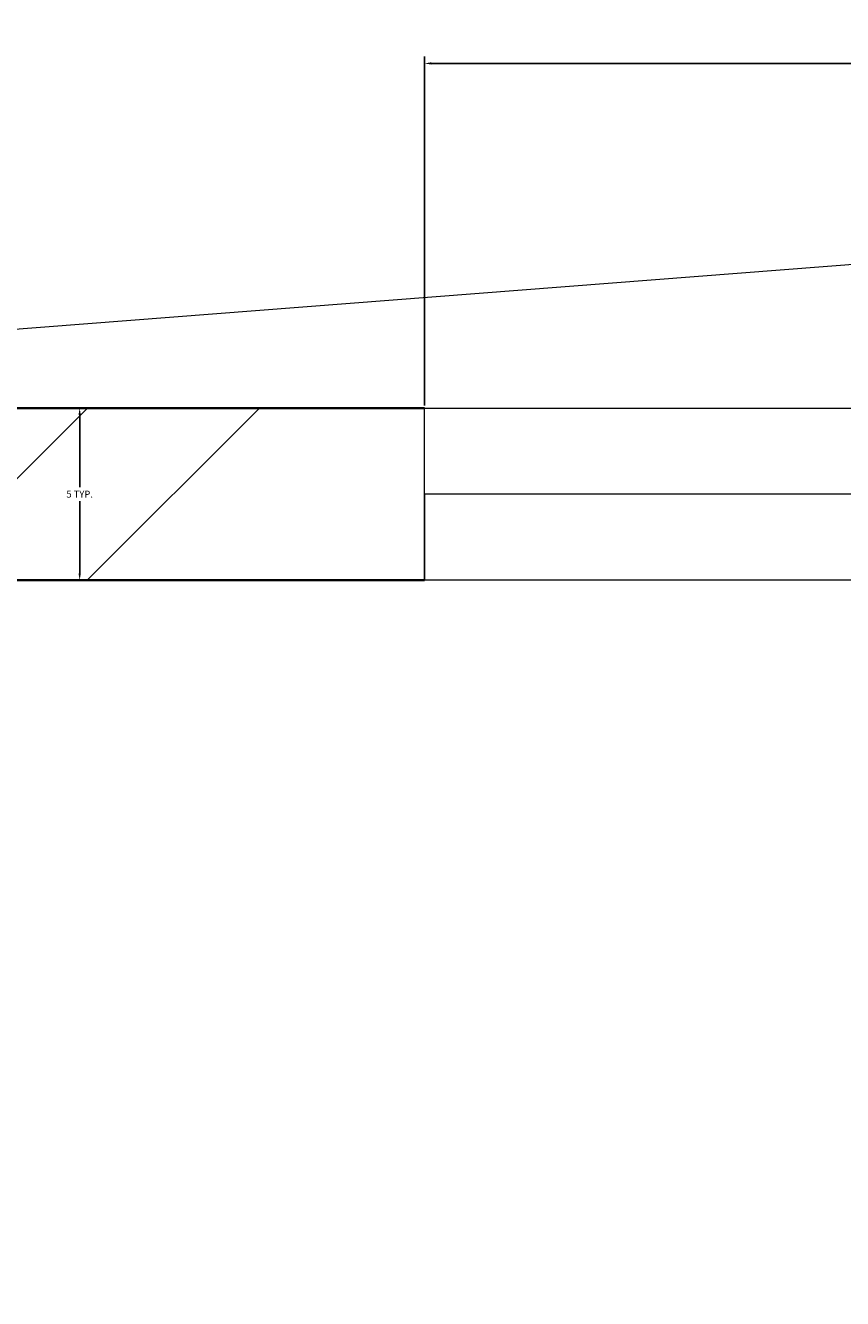
# Model space of a CAD drawing. Units: inches. Extents: x 1885 to 2748, y 783 to 2421.
# Tile 37 of 117: x 2034 to 2056, y 1501 to 1534. Entities that reach past the tile are written whole.
import ezdxf

# ---------------------------------------------------------------- set-up
doc = ezdxf.new("R2010")
doc.units = ezdxf.units.IN
for name, color, linetype, lineweight in [('A-ANNO-DIMS', 2, 'Continuous', 18), ('A-FLOR-OPEN', 8, 'Continuous', 13), ('A-GLAZ', 181, 'Continuous', 18), ('A-WALL', 7, 'Continuous', 35)]:
    doc.layers.add(name, color=color, linetype=linetype, lineweight=lineweight)
doc.layers.add('A-WALL-PATT', color=85, linetype='Continuous', lineweight=13, true_color=0x58ba48)
doc.styles.get("Standard").update_dxf_attribs({"font": 'arial.ttf'})
doc.dimstyles.get("Standard").update_dxf_attribs({"dimtxt": 0.18, "dimasz": 0.18, "dimexe": 0.18, "dimexo": 0.0625, "dimgap": 0.09, "dimtad": 0, "dimtih": 1, "dimtoh": 1, "dimdec": 4, "dimzin": 0, "dimdsep": 46, "dimtxsty": 'Standard', "dimcen": 0.09, "dimadec": 0, "dimazin": 0, "dimtfac": 1, "dimtdec": 4, "dimtofl": 0, "dimtmove": 0, "dimatfit": 3, "dimfxl": 1, "dimtolj": 1, "dimtzin": 0, "dimarcsym": 0})

# ---------------------------------------------------------------- blocks, each defined once
blk = doc.blocks.new('WIN-60')
for p, q in [((0.004, 59.998), (0.004, -0.002)), ((2.254, 59.998), (2.254, -0.002)), ((4.504, -0.002), (4.504, 59.998)), ((2.254, -0.002), (0.004, -0.002)), ((0.004, -0.002), (4.504, -0.002))]:
    blk.add_line(p, q)
blk = doc.blocks.new('*D15')
at = {"layer": 'A-ANNO-DIMS', "color": 0, "lineweight": -2, "transparency": 16777216}
for p, q in [((2044.674, 1524.068), (2044.674, 1533.186)), ((2104.674, 1524.068), (2104.674, 1533.186)), ((2044.854, 1533.006), (2073.556, 1533.006)), ((2104.494, 1533.006), (2075.793, 1533.006))]:
    blk.add_line(p, q, dxfattribs=at)
at = {"layer": 'A-ANNO-DIMS', "color": 0, "transparency": 16777216}
for points in [[(2044.854, 1533.036), (2044.854, 1532.976), (2044.674, 1533.006)], [(2104.494, 1533.036), (2104.494, 1532.976), (2104.674, 1533.006)]]:
    blk.add_solid(points, dxfattribs=at)
at = {"layer": 'Defpoints', "color": 0, "transparency": 16777216}
for p in [(2104.674, 1533.006), (2044.674, 1524.006), (2104.674, 1524.006)]:
    blk.add_point(p, dxfattribs=at)
at = {"layer": 'A-ANNO-DIMS', "color": 0, "transparency": 16777216, "insert": (2074.674, 1533.006), "char_height": 0.18, "attachment_point": 5}
blk.add_mtext('\\A1;WINDOW 60 TYP.', dxfattribs=at)
blk = doc.blocks.new('*D16')
at = {"layer": 'A-ANNO-DIMS', "color": 0, "lineweight": -2, "transparency": 16777216}
for p, q in [((2044.612, 1524.006), (2035.494, 1524.006)), ((2035.674, 1523.826), (2035.674, 1521.937)), ((2035.674, 1519.686), (2035.674, 1521.574)), ((2044.612, 1519.506), (2035.494, 1519.506))]:
    blk.add_line(p, q, dxfattribs=at)
at = {"layer": 'A-ANNO-DIMS', "color": 0, "transparency": 16777216}
for points in [[(2035.644, 1523.826), (2035.704, 1523.826), (2035.674, 1524.006)], [(2035.644, 1519.686), (2035.704, 1519.686), (2035.674, 1519.506)]]:
    blk.add_solid(points, dxfattribs=at)
at = {"layer": 'Defpoints', "color": 0, "transparency": 16777216}
for p in [(2035.674, 1524.006), (2044.674, 1524.006), (2044.674, 1519.506)]:
    blk.add_point(p, dxfattribs=at)
at = {"layer": 'A-ANNO-DIMS', "color": 0, "transparency": 16777216, "insert": (2035.674, 1521.756), "char_height": 0.18, "attachment_point": 5}
blk.add_mtext('\\A1;5 TYP.', dxfattribs=at)

msp = doc.modelspace()

# ---------------------------------------------------------------- hatches: boundary and pattern name
at = {"layer": 'A-WALL-PATT'}
h = msp.add_hatch(dxfattribs=at)
h.set_pattern_fill('ANSI32', color=256)
h.paths.add_polyline_path([(2007.772, 2318.006), (1980.774, 2318.006), (1980.774, 2281.215), (1985.274, 2281.215), (1985.274, 2313.506), (2007.772, 2313.506), (2007.772, 2315.756)])
h.paths.add_polyline_path([(2094.324, 2318.006), (2067.772, 2318.006), (2067.772, 2313.506), (2094.324, 2313.506), (2094.324, 2315.756)])
h.paths.add_polyline_path([(2131.367, 2315.756), (2131.367, 2318.006), (2131.189, 2318.006), (2112.609, 2318.006), (2112.609, 2313.506), (2117.274, 2313.506), (2117.274, 2255.201), (2121.774, 2255.201), (2121.774, 2313.506), (2131.367, 2313.506)])
h.paths.add_polyline_path([(2190.512, 2318.006), (2155.367, 2318.006), (2155.367, 2313.506), (2169.774, 2313.506), (2169.774, 2229.506), (2121.774, 2229.506), (2121.774, 2233.451), (2119.524, 2233.451), (2117.274, 2233.451), (2117.274, 2201.101), (2121.774, 2201.101), (2121.774, 2225.006), (2169.774, 2225.006), (2169.774, 2165.006), (2306.274, 2165.006), (2306.274, 2066.006), (2310.774, 2066.006), (2344.274, 2066.006), (2486.274, 2066.006), (2486.274, 1886.006), (2483.02, 1886.006), (2483.02, 1881.506), (2486.274, 1881.506), (2486.274, 1880.678), (2490.774, 1880.678), (2490.774, 2070.506), (2344.274, 2070.506), (2310.774, 2070.506), (2310.774, 2165.006), (2310.774, 2173.636), (2308.524, 2173.636), (2306.274, 2173.636), (2306.274, 2169.506), (2174.274, 2169.506), (2174.274, 2313.506), (2190.512, 2313.506), (2190.512, 2315.756)])
h.paths.add_polyline_path([(1985.274, 2221.215), (1980.774, 2221.215), (1980.774, 2165.006), (1992.774, 2165.006), (1992.774, 2141.927), (1997.274, 2141.927), (1997.274, 2165.006), (2117.274, 2165.006), (2117.274, 2163.126), (2121.774, 2163.126), (2121.774, 2172.734), (2119.524, 2172.734), (2117.274, 2172.734), (2117.274, 2169.506), (1985.274, 2169.506)])
h.paths.add_polyline_path([(1997.274, 2105.927), (1992.774, 2105.927), (1992.774, 2070.506), (2016.774, 2070.506), (2016.774, 2059.123), (2019.024, 2059.123), (2021.274, 2059.123), (2021.274, 2070.506), (2117.274, 2070.506), (2117.274, 2022.506), (2114.423, 2022.506), (2114.423, 2018.006), (2123.627, 2018.006), (2123.627, 2020.256), (2123.627, 2022.506), (2121.774, 2022.506), (2121.774, 2142.587), (2119.524, 2142.587), (2117.274, 2142.587), (2117.274, 2075.006), (1997.274, 2075.006)])
h.paths.add_polyline_path([(2092.029, 2020.256), (2092.029, 2022.506), (2021.274, 2022.506), (2021.274, 2035.123), (2016.774, 2035.123), (2016.774, 2018.006), (2016.774, 1978.784), (2021.274, 1978.784), (2021.274, 2018.006), (2092.029, 2018.006)])
h.paths.add_polyline_path([(2260.938, 2022.506), (2153.105, 2022.506), (2153.105, 2020.256), (2153.105, 2018.006), (2155.274, 2018.006), (2155.274, 1886.006), (2107.629, 1886.006), (2107.629, 1881.506), (2182.911, 1881.506), (2182.911, 1883.756), (2182.911, 1886.006), (2159.774, 1886.006), (2159.774, 2018.006), (2260.938, 2018.006), (2260.938, 2020.256)])
h.paths.add_polyline_path([(2047.629, 1883.756), (2047.629, 1886.006), (2021.274, 1886.006), (2021.274, 1918.784), (2019.024, 1918.784), (2016.774, 1918.784), (2016.774, 1881.506), (2047.629, 1881.506)])
h.paths.add_polyline_path([(2306.361, 1883.756), (2306.361, 1886.006), (2296.274, 1886.006), (2296.274, 1982.006), (2316.535, 1982.006), (2316.535, 1984.256), (2316.535, 1986.506), (2296.274, 1986.506), (2296.274, 2022.506), (2289.276, 2022.506), (2289.276, 2018.006), (2291.774, 2018.006), (2291.774, 1886.006), (2242.911, 1886.006), (2242.911, 1881.506), (2306.361, 1881.506)], flags=17)
h.paths.add_polyline_path([(1985.274, 1843.006), (2021.6, 1843.006), (2021.534, 1845.441), (2021.477, 1847.506), (1980.774, 1847.506), (1980.774, 1809.446), (1985.274, 1809.446)])
h.paths.add_polyline_path([(2131.482, 1845.256), (2131.482, 1847.506), (2081.534, 1847.506), (2081.534, 1843.006), (2117.274, 1843.006), (2117.274, 1784.147), (2119.524, 1784.147), (2121.774, 1784.147), (2121.774, 1843.006), (2131.482, 1843.006)])
h.paths.add_polyline_path([(2203.886, 1847.506), (2155.482, 1847.506), (2155.482, 1843.006), (2169.774, 1843.006), (2169.774, 1759.006), (2121.774, 1759.006), (2121.774, 1761.457), (2117.274, 1761.457), (2117.274, 1730.429), (2121.774, 1730.429), (2121.774, 1754.506), (2177.421, 1754.506), (2177.421, 1756.756), (2177.421, 1759.006), (2174.274, 1759.006), (2174.274, 1843.006), (2203.886, 1843.006)])
h.paths.add_polyline_path([(2335.554, 1845.256), (2335.554, 1847.506), (2239.886, 1847.506), (2239.886, 1843.006), (2306.274, 1843.006), (2306.274, 1759.006), (2199.486, 1759.006), (2199.486, 1754.506), (2310.774, 1754.506), (2310.774, 1843.006), (2335.554, 1843.006)])
h.paths.add_polyline_path([(2348.774, 2022.506), (2344.274, 2022.506), (2344.274, 1986.506), (2341.681, 1986.506), (2341.681, 1982.006), (2344.274, 1982.006), (2344.274, 1886.006), (2330.361, 1886.006), (2330.361, 1881.506), (2361.627, 1881.506), (2361.627, 1883.756), (2361.627, 1886.006), (2348.774, 1886.006)], flags=17)
h.paths.add_polyline_path([(2283.251, 2315.756), (2283.251, 2318.006), (2238.512, 2318.006), (2238.512, 2313.506), (2283.251, 2313.506)], flags=17)
h.paths.add_polyline_path([(2363.274, 2348.006), (2388.677, 2348.006), (2388.677, 2350.256), (2388.677, 2352.506), (2358.774, 2352.506), (2358.774, 2348.006), (2358.774, 2318.006), (2344.481, 2318.006), (2344.481, 2313.506), (2358.774, 2313.506), (2358.774, 2229.506), (2310.774, 2229.506), (2310.774, 2231.952), (2306.274, 2231.952), (2306.274, 2205.611), (2310.774, 2205.611), (2310.774, 2225.006), (2358.774, 2225.006), (2358.774, 2211.506), (2452.329, 2211.506), (2452.329, 2213.756), (2452.329, 2216.006), (2363.274, 2216.006), (2363.274, 2318.006)])
h.paths.add_polyline_path([(2310.774, 2313.506), (2320.481, 2313.506), (2320.481, 2315.756), (2320.481, 2318.006), (2302.728, 2318.006), (2302.728, 2313.506), (2306.274, 2313.506), (2306.274, 2251.076), (2310.774, 2251.076)], flags=17)
h.paths.add_polyline_path([(2490.774, 2352.506), (2486.274, 2352.506), (2448.677, 2352.506), (2448.677, 2348.006), (2486.274, 2348.006), (2486.274, 2318.006), (2486.274, 2216.006), (2481.78, 2216.006), (2481.78, 2211.506), (2486.274, 2211.506), (2486.274, 2165.006), (2493.289, 2165.006), (2493.289, 2167.256), (2493.289, 2169.506), (2490.774, 2169.506), (2490.774, 2313.506), (2494.429, 2313.506), (2494.429, 2318.006), (2490.774, 2318.006)])
h.paths.add_polyline_path([(2534.653, 2318.006), (2515.691, 2318.006), (2515.691, 2313.506), (2534.653, 2313.506), (2534.653, 2315.756)])
h.paths.add_polyline_path([(2618.274, 2318.006), (2594.653, 2318.006), (2594.653, 2313.506), (2613.774, 2313.506), (2613.774, 2281.706), (2618.274, 2281.706)])
h.paths.add_polyline_path([(2618.274, 2221.706), (2613.774, 2221.706), (2613.774, 2169.506), (2554.019, 2169.506), (2554.019, 2165.006), (2613.774, 2165.006), (2613.774, 2152.878), (2618.274, 2152.878)])
h.paths.add_polyline_path([(2618.274, 2128.878), (2616.024, 2128.878), (2613.774, 2128.878), (2613.774, 2117.006), (2529.774, 2117.006), (2529.774, 2165.006), (2532.848, 2165.006), (2532.848, 2169.506), (2522.867, 2169.506), (2522.867, 2165.006), (2525.274, 2165.006), (2525.274, 2117.006), (2525.274, 2112.506), (2525.274, 2108.576), (2529.774, 2108.576), (2529.774, 2112.506), (2613.774, 2112.506), (2613.774, 2080.19), (2618.274, 2080.19)])
h.paths.add_polyline_path([(2618.274, 2044.19), (2616.024, 2044.19), (2613.774, 2044.19), (2613.774, 2015.506), (2529.774, 2015.506), (2529.774, 2088.582), (2527.524, 2088.582), (2525.274, 2088.582), (2525.274, 2011.006), (2613.774, 2011.006), (2613.774, 1956.755), (2618.274, 1956.755)])
h.paths.add_polyline_path([(2618.274, 1881.506), (2618.274, 1896.755), (2613.774, 1896.755), (2613.774, 1881.506), (2613.774, 1847.506), (2592.715, 1847.506), (2592.715, 1843.006), (2613.774, 1843.006), (2613.774, 1765.006), (2613.774, 1760.506), (2609.621, 1760.506), (2609.621, 1756.006), (2613.774, 1756.006), (2613.774, 1660.006), (2608.544, 1660.006), (2608.544, 1655.506), (2613.774, 1655.506), (2613.774, 1508.158), (2618.274, 1508.158)])
h.paths.add_polyline_path([(2565.774, 1843.006), (2568.997, 1843.006), (2568.997, 1847.506), (2490.774, 1847.506), (2490.774, 1849.7), (2488.524, 1849.7), (2486.274, 1849.7), (2486.274, 1847.506), (2477.274, 1847.506), (2477.274, 1838.506), (2477.274, 1821.493), (2486.274, 1821.493), (2486.274, 1838.506), (2561.274, 1838.506), (2561.274, 1765.006), (2486.274, 1765.006), (2486.274, 1786.157), (2477.274, 1786.157), (2477.274, 1765.006), (2477.274, 1756.006), (2486.274, 1756.006), (2565.774, 1756.006), (2585.621, 1756.006), (2585.621, 1758.256), (2585.621, 1760.506), (2565.774, 1760.506), (2565.774, 1765.006)])
h.paths.add_polyline_path([(2486.274, 1651.006), (2561.274, 1651.006), (2561.274, 1567.006), (2486.274, 1567.006), (2486.274, 1591.321), (2477.274, 1591.321), (2477.274, 1567.006), (2477.274, 1558.006), (2477.274, 1555.439), (2481.774, 1555.439), (2481.774, 1558.006), (2568.653, 1558.006), (2568.653, 1560.256), (2568.653, 1562.506), (2565.774, 1562.506), (2565.774, 1655.506), (2584.544, 1655.506), (2584.544, 1657.756), (2584.544, 1660.006), (2565.774, 1660.006), (2486.274, 1660.006), (2477.274, 1660.006), (2477.274, 1651.006), (2477.274, 1632.989), (2486.274, 1632.989)])
h.paths.add_polyline_path([(2449.967, 1883.756), (2449.967, 1886.006), (2421.627, 1886.006), (2421.627, 1881.506), (2449.967, 1881.506)], flags=17)
h.paths.add_polyline_path([(2447.274, 1847.506), (2395.554, 1847.506), (2395.554, 1843.006), (2442.774, 1843.006), (2442.774, 1809.27), (2447.274, 1809.27)])
h.paths.add_polyline_path([(1985.274, 1749.446), (1980.774, 1749.446), (1980.774, 1694.504), (1985.274, 1694.504), (1985.274, 1694.506), (1986.897, 1694.506), (1986.897, 1697.78), (1986.897, 1699.006), (1985.274, 1699.006)])
h.paths.add_polyline_path([(2152.774, 1699.006), (2121.774, 1699.006), (2121.774, 1703.668), (2119.524, 1703.668), (2117.274, 1703.668), (2117.274, 1699.006), (2009.219, 1699.006), (2009.219, 1694.506), (2148.274, 1694.506), (2148.274, 1692.631), (2152.774, 1692.631)])
h.paths.add_polyline_path([(2016.274, 1694.506), (2011.774, 1694.506), (2011.774, 1558.006), (2040.806, 1558.006), (2040.806, 1560.256), (2040.806, 1562.506), (2016.274, 1562.506)])
h.paths.add_polyline_path([(2152.774, 1663.017), (2150.524, 1663.017), (2148.274, 1663.017), (2148.274, 1562.506), (2100.806, 1562.506), (2100.806, 1558.006), (2165.119, 1558.006), (2165.119, 1560.256), (2165.119, 1562.506), (2152.774, 1562.506), (2152.774, 1610.506), (2224.774, 1610.506), (2224.774, 1607.99), (2229.274, 1607.99), (2229.274, 1615.006), (2152.774, 1615.006)])
h.paths.add_polyline_path([(2238.613, 1560.256), (2238.613, 1562.506), (2229.274, 1562.506), (2229.274, 1588.756), (2227.024, 1588.763), (2224.774, 1588.771), (2224.774, 1562.506), (2189.119, 1562.506), (2189.119, 1558.006), (2238.613, 1558.006)])
h.paths.add_polyline_path([(2336.024, 1560.256), (2336.024, 1562.506), (2310.774, 1562.506), (2310.774, 1656.347), (2308.524, 1656.347), (2306.274, 1656.347), (2306.274, 1562.506), (2286.613, 1562.506), (2286.613, 1558.006), (2336.024, 1558.006)])
h.paths.add_polyline_path([(2447.274, 1690.968), (2445.024, 1690.968), (2442.774, 1690.968), (2442.774, 1687.006), (2306.274, 1687.006), (2306.274, 1680.75), (2310.774, 1680.75), (2310.774, 1682.506), (2442.774, 1682.506), (2442.774, 1562.506), (2396.024, 1562.506), (2396.024, 1558.006), (2447.274, 1558.006)])
h.paths.add_polyline_path([(2447.274, 1749.27), (2445.024, 1749.27), (2442.774, 1749.27), (2442.774, 1717.232), (2447.274, 1717.232)])
h.paths.add_polyline_path([(2044.674, 1521.756), (2044.674, 1524.006), (2007.274, 1524.006), (2007.274, 1503.49), (2009.524, 1503.49), (2011.774, 1503.49), (2011.774, 1519.506), (2044.674, 1519.506)])
h.paths.add_polyline_path([(2177.969, 1521.756), (2177.969, 1524.006), (2104.674, 1524.006), (2104.674, 1519.506), (2145.774, 1519.506), (2145.774, 1387.506), (2143.37, 1387.506), (2143.37, 1383.006), (2251.585, 1383.006), (2251.585, 1385.256), (2251.585, 1387.506), (2150.274, 1387.506), (2150.274, 1519.506), (2177.969, 1519.506)])
h.paths.add_polyline_path([(2298.704, 1524.006), (2237.969, 1524.006), (2237.969, 1519.506), (2282.274, 1519.506), (2282.274, 1387.506), (2279.683, 1387.506), (2279.683, 1383.006), (2286.774, 1383.006), (2286.774, 1419.006), (2312.451, 1419.006), (2312.451, 1421.256), (2312.451, 1423.506), (2286.774, 1423.506), (2286.774, 1519.506), (2298.704, 1519.506), (2298.704, 1521.722)], flags=17)
h.paths.add_polyline_path([(2361.897, 1521.756), (2361.897, 1524.006), (2322.704, 1524.006), (2322.704, 1519.506), (2334.774, 1519.506), (2334.774, 1423.506), (2331.93, 1423.506), (2331.93, 1419.006), (2334.774, 1419.006), (2334.774, 1387.506), (2334.774, 1383.228), (2339.274, 1383.228), (2339.274, 1387.506), (2339.274, 1519.506), (2361.897, 1519.506)], flags=17)
h.paths.add_polyline_path([(2447.274, 1521.756), (2447.274, 1524.006), (2421.897, 1524.006), (2421.897, 1519.506), (2447.274, 1519.506)], flags=17)
h.paths.add_polyline_path([(2481.774, 1529.6), (2479.524, 1529.6), (2477.274, 1529.6), (2477.274, 1524.006), (2474.489, 1524.006), (2474.489, 1519.506), (2477.274, 1519.506), (2477.274, 1334.506), (2296.774, 1334.506), (2296.774, 1240.506), (2160.274, 1240.506), (2160.274, 1180.506), (2112.274, 1180.506), (2112.274, 1207.692), (2110.024, 1207.692), (2107.774, 1207.692), (2107.774, 1171.609), (2112.274, 1171.609), (2112.274, 1176.006), (2160.274, 1176.006), (2160.274, 1092.006), (2144.221, 1092.006), (2144.221, 1087.506), (2189.497, 1087.506), (2189.497, 1089.756), (2189.497, 1092.006), (2164.774, 1092.006), (2164.774, 1236.006), (2296.774, 1236.006), (2296.774, 1231.912), (2301.274, 1231.912), (2301.274, 1330.006), (2481.774, 1330.006), (2481.774, 1387.506)])
h.paths.add_polyline_path([(2618.274, 1448.158), (2613.774, 1448.158), (2613.774, 1382.506), (2529.774, 1382.506), (2525.274, 1382.506), (2525.274, 1307.062), (2529.774, 1307.062), (2529.774, 1378.006), (2613.774, 1378.006), (2613.774, 1354.988), (2618.274, 1354.988)])
h.paths.add_polyline_path([(2618.274, 1318.988), (2613.774, 1318.988), (2613.774, 1281.006), (2529.774, 1281.006), (2529.774, 1283.786), (2527.524, 1283.786), (2525.274, 1283.786), (2525.274, 1228.506), (2516.794, 1228.506), (2516.794, 1224.006), (2533.484, 1224.006), (2533.484, 1226.256), (2533.484, 1228.506), (2529.774, 1228.506), (2529.774, 1276.506), (2613.774, 1276.506), (2613.774, 1266.02), (2618.274, 1266.02)])
h.paths.add_polyline_path([(2618.274, 1134.964), (2613.774, 1134.964), (2613.774, 1092.006), (2594.545, 1092.006), (2594.545, 1087.506), (2618.274, 1087.506)])
h.paths.add_polyline_path([(2534.545, 1092.006), (2509.765, 1092.006), (2509.765, 1087.506), (2534.545, 1087.506), (2534.545, 1089.756)])
h.paths.add_polyline_path([(2481.274, 1224.006), (2484.117, 1224.006), (2484.117, 1226.256), (2484.117, 1228.506), (2476.774, 1228.506), (2476.774, 1198.506), (2471.61, 1198.506), (2471.61, 1194.006), (2476.774, 1194.006), (2476.774, 1062.006), (2436.894, 1062.006), (2436.894, 1057.506), (2476.774, 1057.506), (2481.274, 1057.506), (2481.274, 1062.006), (2481.274, 1087.506), (2485.354, 1087.506), (2485.354, 1089.756), (2485.354, 1092.006), (2481.274, 1092.006), (2481.274, 1117.506)])
h.paths.add_polyline_path([(2439.898, 1198.506), (2349.274, 1198.506), (2349.274, 1194.006), (2349.274, 1180.506), (2301.274, 1180.506), (2301.274, 1201.896), (2299.024, 1201.896), (2296.774, 1201.896), (2296.774, 1172.335), (2299.024, 1172.335), (2301.274, 1172.335), (2301.274, 1176.006), (2349.274, 1176.006), (2349.274, 1092.006), (2334.452, 1092.006), (2334.452, 1087.506), (2349.274, 1087.506), (2349.274, 1057.506), (2353.774, 1057.506), (2376.894, 1057.506), (2376.894, 1059.756), (2376.894, 1062.006), (2353.774, 1062.006), (2353.774, 1087.506), (2353.774, 1180.506), (2353.774, 1194.006), (2439.898, 1194.006), (2439.898, 1196.256)])
h.paths.add_polyline_path([(2270.596, 1089.756), (2270.596, 1092.006), (2249.497, 1092.006), (2249.497, 1087.506), (2270.596, 1087.506)], flags=17)
h.paths.add_polyline_path([(2310.452, 1092.006), (2301.274, 1092.006), (2301.274, 1153.292), (2296.774, 1153.292), (2296.774, 1092.006), (2293.786, 1092.006), (2293.786, 1087.506), (2310.452, 1087.506), (2310.452, 1089.756)], flags=17)
h.paths.add_polyline_path([(2112.274, 1150.328), (2110.024, 1150.328), (2107.774, 1150.328), (2107.774, 1092.006), (2104.465, 1092.006), (2104.465, 1087.506), (2120.221, 1087.506), (2120.221, 1089.756), (2120.221, 1092.006), (2112.274, 1092.006)])
h.paths.add_polyline_path([(2082.172, 1092.006), (2058.144, 1092.006), (2058.144, 1087.506), (2082.172, 1087.506), (2082.172, 1089.756)])
h.paths.add_polyline_path([(1975.774, 1145.638), (1971.274, 1145.638), (1971.274, 1087.506), (1980.774, 1087.506), (1998.144, 1087.506), (1998.144, 1089.756), (1998.144, 1092.006), (1985.274, 1092.006), (1975.774, 1092.006)])
h.paths.add_polyline_path([(2112.274, 1244.385), (2110.024, 1244.385), (2107.774, 1244.385), (2107.774, 1240.506), (1992.274, 1240.506), (1992.274, 1271.008), (1987.774, 1271.008), (1987.774, 1240.506), (1980.774, 1240.506), (1975.774, 1240.506), (1971.274, 1240.506), (1971.274, 1205.638), (1975.774, 1205.638), (1975.774, 1236.006), (2107.774, 1236.006), (2107.774, 1233.444), (2112.274, 1233.444), (2112.274, 1236.006)])
h.paths.add_polyline_path([(2112.274, 1383.006), (2114.783, 1383.006), (2114.783, 1385.256), (2114.783, 1387.506), (2102.476, 1387.506), (2102.476, 1383.006), (2107.774, 1383.006), (2107.774, 1335.006), (2011.774, 1335.006), (2011.774, 1349.939), (2007.274, 1349.939), (2007.274, 1335.006), (1987.774, 1335.006), (1987.774, 1330.506), (1987.774, 1307.008), (1992.274, 1307.008), (1992.274, 1330.506), (2007.274, 1330.506), (2107.774, 1330.506), (2107.774, 1264.711), (2112.274, 1264.711)])
h.paths.add_polyline_path([(2077.857, 1387.506), (2011.774, 1387.506), (2011.774, 1390.036), (2009.524, 1390.036), (2007.274, 1390.036), (2007.274, 1373.939), (2011.774, 1373.939), (2011.774, 1383.006), (2077.857, 1383.006)])
h.paths.add_polyline_path([(2011.774, 1443.49), (2007.274, 1443.49), (2007.274, 1410.248), (2011.774, 1410.248)])

# ---------------------------------------------------------------- linework, layer by layer
at = {"layer": 'A-FLOR-OPEN'}
msp.add_line((2007.274, 1524.006), (2447.274, 1558.006), dxfattribs=at)
at = {"layer": 'A-WALL'}
for p, q in [((1980.774, 1524.006), (2044.674, 1524.006)), ((2011.774, 1519.506), (2044.674, 1519.506))]:
    msp.add_line(p, q, dxfattribs=at)

# ---------------------------------------------------------------- block references
at = {"layer": 'A-GLAZ', "extrusion": (0, 0, -1), "zscale": -1, "rotation": 90}
msp.add_blockref('WIN-60', (-2044.676, 1519.502), dxfattribs=at)

# ---------------------------------------------------------------- dimensions: what is measured, and where the dimension line sits
at = {"layer": 'A-ANNO-DIMS'}
dim = msp.add_linear_dim(base=(2104.674, 1533.006), p1=(2044.674, 1524.006), p2=(2104.674, 1524.006), text='WINDOW <> TYP.', dimstyle='Standard', override={"dimdec": 0, "dimlfac": 1, "dimrnd": 0, "dimzin": 0, "dimdsep": 46, "dimlunit": 2}, dxfattribs=at)
dim.commit()
dim.dimension.update_dxf_attribs({"geometry": '*D15', "text_midpoint": (2074.674, 1533.006)})
dim = msp.add_linear_dim(base=(2035.674185368, 1524.005556822), p1=(2044.674185368, 1519.505556822), p2=(2044.674185368, 1524.005556822), angle=90, text='<> TYP.', dimstyle='Standard', override={"dimdec": 0, "dimlfac": 1, "dimrnd": 0, "dimzin": 0, "dimdsep": 46, "dimlunit": 2}, dxfattribs=at)
dim.commit()
dim.dimension.update_dxf_attribs({"geometry": '*D16', "text_midpoint": (2035.674185368, 1521.755556822)})

doc.saveas('drawing.dxf')
